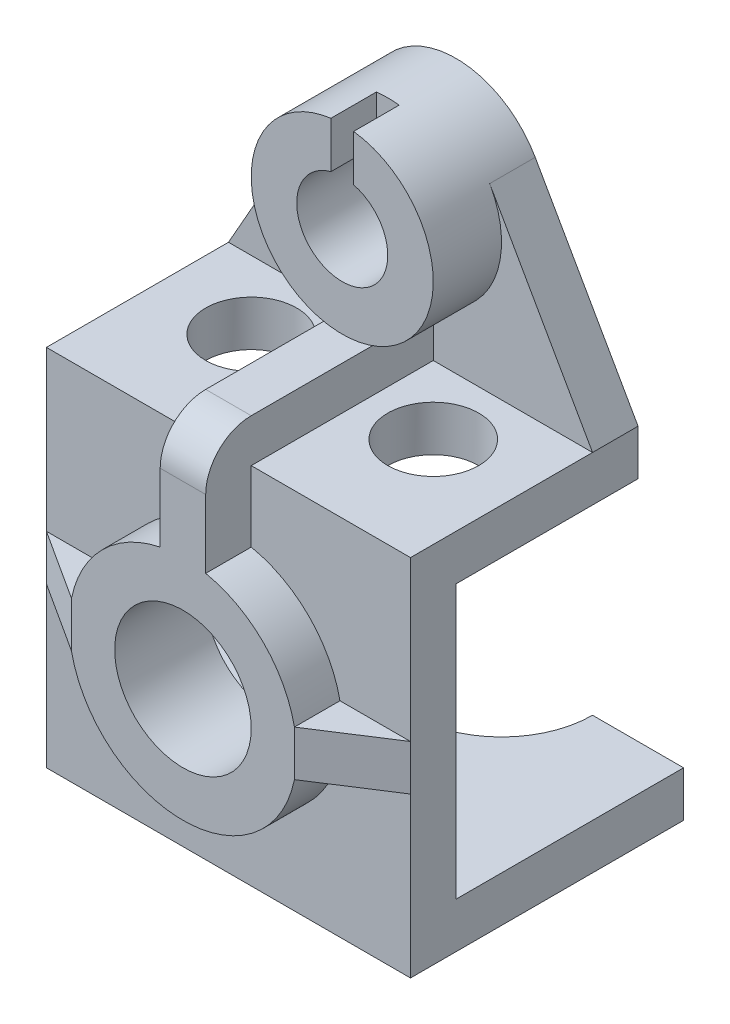
ISO-10303-21;
HEADER;
FILE_DESCRIPTION(('STEP AP214'),'2;1');
FILE_NAME('part.step','',(''),(''),'','','');
FILE_SCHEMA(('AUTOMOTIVE_DESIGN { 1 0 10303 214 1 1 1 1 }'));
ENDSEC;
DATA;
#1=APPLICATION_CONTEXT('core data for automotive mechanical design processes');
#2=APPLICATION_PROTOCOL_DEFINITION('international standard','automotive_design',2000,#1);
#3=PRODUCT_CONTEXT('',#1,'mechanical');
#4=PRODUCT('Part','Part','',(#3));
#5=PRODUCT_RELATED_PRODUCT_CATEGORY('part','',(#4));
#6=PRODUCT_DEFINITION_FORMATION('','',#4);
#7=PRODUCT_DEFINITION_CONTEXT('part definition',#1,'design');
#8=PRODUCT_DEFINITION('design','',#6,#7);
#9=PRODUCT_DEFINITION_SHAPE('','',#8);
#10=(LENGTH_UNIT() NAMED_UNIT(*) SI_UNIT(.MILLI.,.METRE.));
#11=(NAMED_UNIT(*) PLANE_ANGLE_UNIT() SI_UNIT($,.RADIAN.));
#12=(NAMED_UNIT(*) SI_UNIT($,.STERADIAN.) SOLID_ANGLE_UNIT());
#13=UNCERTAINTY_MEASURE_WITH_UNIT(LENGTH_MEASURE(1.E-05),#10,'distance_accuracy_value','');
#14=(GEOMETRIC_REPRESENTATION_CONTEXT(3) GLOBAL_UNCERTAINTY_ASSIGNED_CONTEXT((#13)) GLOBAL_UNIT_ASSIGNED_CONTEXT((#10,
#11,#12)) REPRESENTATION_CONTEXT('',''));
#15=CARTESIAN_POINT('',(0.,0.,0.));
#16=DIRECTION('',(0.,0.,1.));
#17=DIRECTION('',(1.,0.,0.));
#18=AXIS2_PLACEMENT_3D('',#15,#16,#17);
#19=CARTESIAN_POINT('',(-80.,9.99999999999999,0.));
#20=DIRECTION('',(0.,0.,-1.));
#21=DIRECTION('',(-1.,0.,0.));
#22=AXIS2_PLACEMENT_3D('',#19,#20,#21);
#23=PLANE('',#22);
#24=DIRECTION('',(0.,1.,0.));
#25=VECTOR('',#24,1.);
#26=CARTESIAN_POINT('',(-60.,0.,0.));
#27=LINE('',#26,#25);
#28=CARTESIAN_POINT('',(-60.,0.,0.));
#29=VERTEX_POINT('',#28);
#30=CARTESIAN_POINT('',(-60.,9.99999999999999,0.));
#31=VERTEX_POINT('',#30);
#32=EDGE_CURVE('E56',#29,#31,#27,.T.);
#33=ORIENTED_EDGE('',*,*,#32,.F.);
#34=DIRECTION('',(1.,0.,0.));
#35=VECTOR('',#34,1.);
#36=CARTESIAN_POINT('',(-80.,0.,0.));
#37=LINE('',#36,#35);
#38=CARTESIAN_POINT('',(-80.,0.,0.));
#39=VERTEX_POINT('',#38);
#40=EDGE_CURVE('E251',#39,#29,#37,.T.);
#41=ORIENTED_EDGE('',*,*,#40,.F.);
#42=DIRECTION('',(0.,1.,0.));
#43=VECTOR('',#42,1.);
#44=CARTESIAN_POINT('',(-80.,9.99999999999999,0.));
#45=LINE('',#44,#43);
#46=CARTESIAN_POINT('',(-80.,9.99999999999999,0.));
#47=VERTEX_POINT('',#46);
#48=EDGE_CURVE('E425',#39,#47,#45,.T.);
#49=ORIENTED_EDGE('',*,*,#48,.T.);
#50=DIRECTION('',(1.,0.,0.));
#51=VECTOR('',#50,1.);
#52=CARTESIAN_POINT('',(-80.,9.99999999999999,0.));
#53=LINE('',#52,#51);
#54=EDGE_CURVE('E276',#47,#31,#53,.T.);
#55=ORIENTED_EDGE('',*,*,#54,.T.);
#56=EDGE_LOOP('',(#33,#41,#49,#55));
#57=FACE_BOUND('',#56,.T.);
#58=ADVANCED_FACE('F44',(#57),#23,.T.);
#59=CARTESIAN_POINT('',(-40.,110.,35.));
#60=DIRECTION('',(0.,0.,-1.));
#61=DIRECTION('',(-1.,0.,0.));
#62=AXIS2_PLACEMENT_3D('',#59,#60,#61);
#63=CYLINDRICAL_SURFACE('',#62,20.);
#64=DIRECTION('',(0.,0.,-1.));
#65=VECTOR('',#64,1.);
#66=CARTESIAN_POINT('',(-57.398181667894,119.864242223859,20.));
#67=LINE('',#66,#65);
#68=CARTESIAN_POINT('',(-57.398181667894,119.864242223859,20.));
#69=VERTEX_POINT('',#68);
#70=CARTESIAN_POINT('',(-57.398181667894,119.864242223859,9.99999999999999));
#71=VERTEX_POINT('',#70);
#72=EDGE_CURVE('E415',#69,#71,#67,.T.);
#73=ORIENTED_EDGE('',*,*,#72,.F.);
#74=CARTESIAN_POINT('',(-40.,110.,20.));
#75=DIRECTION('',(0.,0.,-1.));
#76=DIRECTION('',(-1.,0.,0.));
#77=AXIS2_PLACEMENT_3D('',#74,#75,#76);
#78=CIRCLE('',#77,20.);
#79=CARTESIAN_POINT('',(-22.601818332106,119.864242223859,20.));
#80=VERTEX_POINT('',#79);
#81=EDGE_CURVE('E393',#80,#69,#78,.T.);
#82=ORIENTED_EDGE('',*,*,#81,.F.);
#83=DIRECTION('',(0.,0.,-1.));
#84=VECTOR('',#83,1.);
#85=CARTESIAN_POINT('',(-22.601818332106,119.864242223859,20.));
#86=LINE('',#85,#84);
#87=CARTESIAN_POINT('',(-22.601818332106,119.864242223859,9.99999999999999));
#88=VERTEX_POINT('',#87);
#89=EDGE_CURVE('E410',#80,#88,#86,.T.);
#90=ORIENTED_EDGE('',*,*,#89,.T.);
#91=CARTESIAN_POINT('',(-40.,110.,9.99999999999999));
#92=DIRECTION('',(0.,0.,-1.));
#93=DIRECTION('',(-1.,0.,0.));
#94=AXIS2_PLACEMENT_3D('',#91,#92,#93);
#95=CIRCLE('',#94,20.);
#96=EDGE_CURVE('E380',#71,#88,#95,.T.);
#97=ORIENTED_EDGE('',*,*,#96,.F.);
#98=EDGE_LOOP('',(#73,#82,#90,#97));
#99=FACE_BOUND('',#98,.T.);
#100=CARTESIAN_POINT('',(-40.,110.,35.));
#101=DIRECTION('',(0.,0.,-1.));
#102=DIRECTION('',(-1.,0.,0.));
#103=AXIS2_PLACEMENT_3D('',#100,#101,#102);
#104=CIRCLE('',#103,20.);
#105=CARTESIAN_POINT('',(-37.5000000000001,129.843134832984,35.));
#106=VERTEX_POINT('',#105);
#107=CARTESIAN_POINT('',(-42.5,129.843134832984,35.));
#108=VERTEX_POINT('',#107);
#109=EDGE_CURVE('E390',#106,#108,#104,.T.);
#110=ORIENTED_EDGE('',*,*,#109,.T.);
#111=DIRECTION('',(0.,0.,1.));
#112=VECTOR('',#111,1.);
#113=CARTESIAN_POINT('',(-42.5,129.843134832984,25.));
#114=LINE('',#113,#112);
#115=CARTESIAN_POINT('',(-42.5,129.843134832984,25.));
#116=VERTEX_POINT('',#115);
#117=EDGE_CURVE('E506',#116,#108,#114,.T.);
#118=ORIENTED_EDGE('',*,*,#117,.F.);
#119=CARTESIAN_POINT('',(-40.,110.,25.));
#120=DIRECTION('',(0.,0.,1.));
#121=DIRECTION('',(1.,0.,0.));
#122=AXIS2_PLACEMENT_3D('',#119,#120,#121);
#123=CIRCLE('',#122,20.);
#124=CARTESIAN_POINT('',(-37.5000000000001,129.843134832984,25.));
#125=VERTEX_POINT('',#124);
#126=EDGE_CURVE('E496',#125,#116,#123,.T.);
#127=ORIENTED_EDGE('',*,*,#126,.F.);
#128=DIRECTION('',(0.,0.,1.));
#129=VECTOR('',#128,1.);
#130=CARTESIAN_POINT('',(-37.5000000000001,129.843134832984,25.));
#131=LINE('',#130,#129);
#132=EDGE_CURVE('E507',#125,#106,#131,.T.);
#133=ORIENTED_EDGE('',*,*,#132,.T.);
#134=EDGE_LOOP('',(#110,#118,#127,#133));
#135=FACE_BOUND('',#134,.T.);
#136=ADVANCED_FACE('F566',(#99,#135),#63,.T.);
#137=CARTESIAN_POINT('',(0.,0.,35.));
#138=DIRECTION('',(0.,0.,-1.));
#139=DIRECTION('',(-1.,0.,0.));
#140=AXIS2_PLACEMENT_3D('',#137,#138,#139);
#141=PLANE('',#140);
#142=DIRECTION('',(0.,1.,0.));
#143=VECTOR('',#142,1.);
#144=CARTESIAN_POINT('',(-42.5000000000002,0.,35.));
#145=LINE('',#144,#143);
#146=CARTESIAN_POINT('',(-42.5,119.682458365519,35.));
#147=VERTEX_POINT('',#146);
#148=EDGE_CURVE('E487',#147,#108,#145,.T.);
#149=ORIENTED_EDGE('',*,*,#148,.T.);
#150=ORIENTED_EDGE('',*,*,#109,.F.);
#151=DIRECTION('',(0.,1.,0.));
#152=VECTOR('',#151,1.);
#153=CARTESIAN_POINT('',(-37.4999999999997,-1.02437479327167E-13,35.));
#154=LINE('',#153,#152);
#155=CARTESIAN_POINT('',(-37.5,119.682458365519,35.));
#156=VERTEX_POINT('',#155);
#157=EDGE_CURVE('E481',#156,#106,#154,.T.);
#158=ORIENTED_EDGE('',*,*,#157,.F.);
#159=CARTESIAN_POINT('',(-40.,110.,35.));
#160=DIRECTION('',(0.,0.,1.));
#161=DIRECTION('',(1.,0.,0.));
#162=AXIS2_PLACEMENT_3D('',#159,#160,#161);
#163=CIRCLE('',#162,10.);
#164=EDGE_CURVE('E504',#147,#156,#163,.T.);
#165=ORIENTED_EDGE('',*,*,#164,.F.);
#166=EDGE_LOOP('',(#149,#150,#158,#165));
#167=FACE_BOUND('',#166,.T.);
#168=ADVANCED_FACE('F637',(#167),#141,.F.);
#169=CARTESIAN_POINT('',(-40.,110.,0.));
#170=DIRECTION('',(0.,0.,1.));
#171=DIRECTION('',(1.,0.,0.));
#172=AXIS2_PLACEMENT_3D('',#169,#170,#171);
#173=CYLINDRICAL_SURFACE('',#172,10.);
#174=CARTESIAN_POINT('',(-40.,110.,9.99999999999999));
#175=DIRECTION('',(0.,0.,-1.));
#176=DIRECTION('',(-1.,0.,0.));
#177=AXIS2_PLACEMENT_3D('',#174,#175,#176);
#178=CIRCLE('',#177,10.);
#179=CARTESIAN_POINT('',(-50.,110.,9.99999999999999));
#180=VERTEX_POINT('',#179);
#181=EDGE_CURVE('E511',#180,#180,#178,.T.);
#182=ORIENTED_EDGE('',*,*,#181,.T.);
#183=EDGE_LOOP('',(#182));
#184=FACE_BOUND('',#183,.T.);
#185=DIRECTION('',(0.,0.,1.));
#186=VECTOR('',#185,1.);
#187=CARTESIAN_POINT('',(-42.5,119.682458365519,25.));
#188=LINE('',#187,#186);
#189=CARTESIAN_POINT('',(-42.5,119.682458365519,25.));
#190=VERTEX_POINT('',#189);
#191=EDGE_CURVE('E70',#190,#147,#188,.T.);
#192=ORIENTED_EDGE('',*,*,#191,.T.);
#193=ORIENTED_EDGE('',*,*,#164,.T.);
#194=DIRECTION('',(0.,0.,1.));
#195=VECTOR('',#194,1.);
#196=CARTESIAN_POINT('',(-37.5,119.682458365519,25.));
#197=LINE('',#196,#195);
#198=CARTESIAN_POINT('',(-37.5,119.682458365519,25.));
#199=VERTEX_POINT('',#198);
#200=EDGE_CURVE('E499',#199,#156,#197,.T.);
#201=ORIENTED_EDGE('',*,*,#200,.F.);
#202=CARTESIAN_POINT('',(-40.,110.,25.));
#203=DIRECTION('',(0.,0.,1.));
#204=DIRECTION('',(1.,0.,0.));
#205=AXIS2_PLACEMENT_3D('',#202,#203,#204);
#206=CIRCLE('',#205,10.);
#207=EDGE_CURVE('E489',#199,#190,#206,.T.);
#208=ORIENTED_EDGE('',*,*,#207,.T.);
#209=EDGE_LOOP('',(#192,#193,#201,#208));
#210=FACE_BOUND('',#209,.T.);
#211=ADVANCED_FACE('F681',(#184,#210),#173,.F.);
#212=CARTESIAN_POINT('',(-80.,0.,60.));
#213=DIRECTION('',(0.,0.,1.));
#214=DIRECTION('',(1.,0.,0.));
#215=AXIS2_PLACEMENT_3D('',#212,#213,#214);
#216=PLANE('',#215);
#217=DIRECTION('',(-1.,0.,0.));
#218=VECTOR('',#217,1.);
#219=CARTESIAN_POINT('',(-64.4948974278318,35.,60.));
#220=LINE('',#219,#218);
#221=CARTESIAN_POINT('',(-64.4948974278318,35.,60.));
#222=VERTEX_POINT('',#221);
#223=CARTESIAN_POINT('',(-80.,35.,60.));
#224=VERTEX_POINT('',#223);
#225=EDGE_CURVE('E340',#222,#224,#220,.T.);
#226=ORIENTED_EDGE('',*,*,#225,.T.);
#227=DIRECTION('',(0.,-1.,0.));
#228=VECTOR('',#227,1.);
#229=CARTESIAN_POINT('',(-80.,0.,60.));
#230=LINE('',#229,#228);
#231=CARTESIAN_POINT('',(-80.,0.,60.));
#232=VERTEX_POINT('',#231);
#233=EDGE_CURVE('E442',#224,#232,#230,.T.);
#234=ORIENTED_EDGE('',*,*,#233,.T.);
#235=DIRECTION('',(1.,0.,0.));
#236=VECTOR('',#235,1.);
#237=CARTESIAN_POINT('',(-80.,0.,60.));
#238=LINE('',#237,#236);
#239=CARTESIAN_POINT('',(0.,0.,60.));
#240=VERTEX_POINT('',#239);
#241=EDGE_CURVE('E258',#232,#240,#238,.T.);
#242=ORIENTED_EDGE('',*,*,#241,.T.);
#243=DIRECTION('',(0.,-1.,0.));
#244=VECTOR('',#243,1.);
#245=CARTESIAN_POINT('',(0.,0.,60.));
#246=LINE('',#245,#244);
#247=CARTESIAN_POINT('',(0.,35.,60.));
#248=VERTEX_POINT('',#247);
#249=EDGE_CURVE('E465',#248,#240,#246,.T.);
#250=ORIENTED_EDGE('',*,*,#249,.F.);
#251=DIRECTION('',(-1.,0.,0.));
#252=VECTOR('',#251,1.);
#253=CARTESIAN_POINT('',(-15.5051025721682,35.,60.));
#254=LINE('',#253,#252);
#255=CARTESIAN_POINT('',(-15.5051025721682,35.,60.));
#256=VERTEX_POINT('',#255);
#257=EDGE_CURVE('E349',#248,#256,#254,.T.);
#258=ORIENTED_EDGE('',*,*,#257,.T.);
#259=CARTESIAN_POINT('',(-40.,40.,60.));
#260=DIRECTION('',(0.,0.,1.));
#261=DIRECTION('',(1.,0.,0.));
#262=AXIS2_PLACEMENT_3D('',#259,#260,#261);
#263=CIRCLE('',#262,25.);
#264=EDGE_CURVE('E421',#222,#256,#263,.T.);
#265=ORIENTED_EDGE('',*,*,#264,.F.);
#266=EDGE_LOOP('',(#226,#234,#242,#250,#258,#265));
#267=FACE_BOUND('',#266,.T.);
#268=ADVANCED_FACE('F477',(#267),#216,.T.);
#269=CARTESIAN_POINT('',(-40.,40.,70.));
#270=DIRECTION('',(0.,0.,-1.));
#271=DIRECTION('',(-1.,0.,0.));
#272=AXIS2_PLACEMENT_3D('',#269,#270,#271);
#273=CYLINDRICAL_SURFACE('',#272,25.);
#274=CARTESIAN_POINT('',(-40.,40.,70.));
#275=DIRECTION('',(0.,0.,1.));
#276=DIRECTION('',(1.,0.,0.));
#277=AXIS2_PLACEMENT_3D('',#274,#275,#276);
#278=CIRCLE('',#277,25.);
#279=CARTESIAN_POINT('',(-64.4948974278318,35.,70.));
#280=VERTEX_POINT('',#279);
#281=CARTESIAN_POINT('',(-15.5051025721682,35.,70.));
#282=VERTEX_POINT('',#281);
#283=EDGE_CURVE('E416',#280,#282,#278,.T.);
#284=ORIENTED_EDGE('',*,*,#283,.F.);
#285=DIRECTION('',(0.,0.,1.));
#286=VECTOR('',#285,1.);
#287=CARTESIAN_POINT('',(-64.4948974278318,35.,-0.002000000000002));
#288=LINE('',#287,#286);
#289=EDGE_CURVE('E329',#222,#280,#288,.T.);
#290=ORIENTED_EDGE('',*,*,#289,.F.);
#291=ORIENTED_EDGE('',*,*,#264,.T.);
#292=DIRECTION('',(0.,0.,1.));
#293=VECTOR('',#292,1.);
#294=CARTESIAN_POINT('',(-15.5051025721682,35.,-0.002000000000002));
#295=LINE('',#294,#293);
#296=EDGE_CURVE('E345',#256,#282,#295,.T.);
#297=ORIENTED_EDGE('',*,*,#296,.T.);
#298=EDGE_LOOP('',(#284,#290,#291,#297));
#299=FACE_BOUND('',#298,.T.);
#300=ADVANCED_FACE('F594',(#299),#273,.T.);
#301=DIRECTION('',(1.,0.,0.));
#302=VECTOR('',#301,1.);
#303=CARTESIAN_POINT('',(-64.4948974278318,45.,60.));
#304=LINE('',#303,#302);
#305=CARTESIAN_POINT('',(-80.,45.,60.));
#306=VERTEX_POINT('',#305);
#307=CARTESIAN_POINT('',(-64.4948974278318,45.,60.));
#308=VERTEX_POINT('',#307);
#309=EDGE_CURVE('E334',#306,#308,#304,.T.);
#310=ORIENTED_EDGE('',*,*,#309,.T.);
#311=CARTESIAN_POINT('',(-45.,64.4948974278318,60.));
#312=VERTEX_POINT('',#311);
#313=EDGE_CURVE('E289',#312,#308,#263,.T.);
#314=ORIENTED_EDGE('',*,*,#313,.F.);
#315=DIRECTION('',(0.,1.,0.));
#316=VECTOR('',#315,1.);
#317=CARTESIAN_POINT('',(-45.,-0.002000000000002,60.));
#318=LINE('',#317,#316);
#319=CARTESIAN_POINT('',(-45.,80.,60.));
#320=VERTEX_POINT('',#319);
#321=EDGE_CURVE('E355',#312,#320,#318,.T.);
#322=ORIENTED_EDGE('',*,*,#321,.T.);
#323=DIRECTION('',(1.,0.,0.));
#324=VECTOR('',#323,1.);
#325=CARTESIAN_POINT('',(-80.,80.,60.));
#326=LINE('',#325,#324);
#327=CARTESIAN_POINT('',(-80.,80.,60.));
#328=VERTEX_POINT('',#327);
#329=EDGE_CURVE('E264',#328,#320,#326,.T.);
#330=ORIENTED_EDGE('',*,*,#329,.F.);
#331=EDGE_CURVE('E443',#328,#306,#230,.T.);
#332=ORIENTED_EDGE('',*,*,#331,.T.);
#333=EDGE_LOOP('',(#310,#314,#322,#330,#332));
#334=FACE_BOUND('',#333,.T.);
#335=ADVANCED_FACE('F608',(#334),#216,.T.);
#336=ORIENTED_EDGE('',*,*,#313,.T.);
#337=DIRECTION('',(0.,0.,1.));
#338=VECTOR('',#337,1.);
#339=CARTESIAN_POINT('',(-64.4948974278318,45.,-0.002000000000002));
#340=LINE('',#339,#338);
#341=CARTESIAN_POINT('',(-64.4948974278318,45.,70.));
#342=VERTEX_POINT('',#341);
#343=EDGE_CURVE('E332',#308,#342,#340,.T.);
#344=ORIENTED_EDGE('',*,*,#343,.T.);
#345=CARTESIAN_POINT('',(-45.,64.4948974278318,70.));
#346=VERTEX_POINT('',#345);
#347=EDGE_CURVE('E419',#346,#342,#278,.T.);
#348=ORIENTED_EDGE('',*,*,#347,.F.);
#349=DIRECTION('',(0.,0.,-1.));
#350=VECTOR('',#349,1.);
#351=CARTESIAN_POINT('',(-45.,64.4948974278318,70.));
#352=LINE('',#351,#350);
#353=EDGE_CURVE('E343',#346,#312,#352,.T.);
#354=ORIENTED_EDGE('',*,*,#353,.T.);
#355=EDGE_LOOP('',(#336,#344,#348,#354));
#356=FACE_BOUND('',#355,.T.);
#357=ADVANCED_FACE('F615',(#356),#273,.T.);
#358=DIRECTION('',(1.,0.,0.));
#359=VECTOR('',#358,1.);
#360=CARTESIAN_POINT('',(-15.5051025721682,45.,60.));
#361=LINE('',#360,#359);
#362=CARTESIAN_POINT('',(-15.5051025721682,45.,60.));
#363=VERTEX_POINT('',#362);
#364=CARTESIAN_POINT('',(0.,45.,60.));
#365=VERTEX_POINT('',#364);
#366=EDGE_CURVE('E347',#363,#365,#361,.T.);
#367=ORIENTED_EDGE('',*,*,#366,.T.);
#368=CARTESIAN_POINT('',(0.,80.,60.));
#369=VERTEX_POINT('',#368);
#370=EDGE_CURVE('E461',#369,#365,#246,.T.);
#371=ORIENTED_EDGE('',*,*,#370,.F.);
#372=CARTESIAN_POINT('',(-35.,80.,60.));
#373=VERTEX_POINT('',#372);
#374=EDGE_CURVE('E275',#373,#369,#326,.T.);
#375=ORIENTED_EDGE('',*,*,#374,.F.);
#376=DIRECTION('',(0.,1.,0.));
#377=VECTOR('',#376,1.);
#378=CARTESIAN_POINT('',(-35.,-0.002000000000002,60.));
#379=LINE('',#378,#377);
#380=CARTESIAN_POINT('',(-35.,64.4948974278318,60.));
#381=VERTEX_POINT('',#380);
#382=EDGE_CURVE('E358',#381,#373,#379,.T.);
#383=ORIENTED_EDGE('',*,*,#382,.F.);
#384=EDGE_CURVE('E265',#363,#381,#263,.T.);
#385=ORIENTED_EDGE('',*,*,#384,.F.);
#386=EDGE_LOOP('',(#367,#371,#375,#383,#385));
#387=FACE_BOUND('',#386,.T.);
#388=ADVANCED_FACE('F572',(#387),#216,.T.);
#389=CARTESIAN_POINT('',(-15.5051025721682,45.,70.));
#390=VERTEX_POINT('',#389);
#391=CARTESIAN_POINT('',(-35.,64.4948974278318,70.));
#392=VERTEX_POINT('',#391);
#393=EDGE_CURVE('E411',#390,#392,#278,.T.);
#394=ORIENTED_EDGE('',*,*,#393,.F.);
#395=DIRECTION('',(0.,0.,1.));
#396=VECTOR('',#395,1.);
#397=CARTESIAN_POINT('',(-15.5051025721682,45.,-0.002000000000002));
#398=LINE('',#397,#396);
#399=EDGE_CURVE('E337',#363,#390,#398,.T.);
#400=ORIENTED_EDGE('',*,*,#399,.F.);
#401=ORIENTED_EDGE('',*,*,#384,.T.);
#402=DIRECTION('',(0.,0.,-1.));
#403=VECTOR('',#402,1.);
#404=CARTESIAN_POINT('',(-35.,64.4948974278318,70.));
#405=LINE('',#404,#403);
#406=EDGE_CURVE('E357',#381,#392,#405,.F.);
#407=ORIENTED_EDGE('',*,*,#406,.T.);
#408=EDGE_LOOP('',(#394,#400,#401,#407));
#409=FACE_BOUND('',#408,.T.);
#410=ADVANCED_FACE('F529',(#409),#273,.T.);
#411=CARTESIAN_POINT('',(-80.,80.,60.));
#412=DIRECTION('',(0.,1.,0.));
#413=DIRECTION('',(0.,0.,1.));
#414=AXIS2_PLACEMENT_3D('',#411,#412,#413);
#415=PLANE('',#414);
#416=CARTESIAN_POINT('',(-60.,80.,35.));
#417=DIRECTION('',(0.,1.,0.));
#418=DIRECTION('',(0.,0.,1.));
#419=AXIS2_PLACEMENT_3D('',#416,#417,#418);
#420=CIRCLE('',#419,10.);
#421=CARTESIAN_POINT('',(-60.,80.,45.));
#422=VERTEX_POINT('',#421);
#423=EDGE_CURVE('E307',#422,#422,#420,.T.);
#424=ORIENTED_EDGE('',*,*,#423,.F.);
#425=EDGE_LOOP('',(#424));
#426=FACE_BOUND('',#425,.T.);
#427=DIRECTION('',(0.,0.,1.));
#428=VECTOR('',#427,1.);
#429=CARTESIAN_POINT('',(-45.,80.,-0.002000000000002));
#430=LINE('',#429,#428);
#431=CARTESIAN_POINT('',(-45.,80.,20.));
#432=VERTEX_POINT('',#431);
#433=EDGE_CURVE('E369',#432,#320,#430,.T.);
#434=ORIENTED_EDGE('',*,*,#433,.F.);
#435=DIRECTION('',(1.,0.,0.));
#436=VECTOR('',#435,1.);
#437=CARTESIAN_POINT('',(0.,80.,20.));
#438=LINE('',#437,#436);
#439=CARTESIAN_POINT('',(-80.,80.,20.));
#440=VERTEX_POINT('',#439);
#441=EDGE_CURVE('E402',#440,#432,#438,.T.);
#442=ORIENTED_EDGE('',*,*,#441,.F.);
#443=DIRECTION('',(0.,0.,1.));
#444=VECTOR('',#443,1.);
#445=CARTESIAN_POINT('',(-80.,80.,60.));
#446=LINE('',#445,#444);
#447=EDGE_CURVE('E437',#440,#328,#446,.T.);
#448=ORIENTED_EDGE('',*,*,#447,.T.);
#449=ORIENTED_EDGE('',*,*,#329,.T.);
#450=EDGE_LOOP('',(#434,#442,#448,#449));
#451=FACE_BOUND('',#450,.T.);
#452=ADVANCED_FACE('F524',(#426,#451),#415,.T.);
#453=DIRECTION('',(0.,1.,0.));
#454=VECTOR('',#453,1.);
#455=CARTESIAN_POINT('',(-20.,0.,0.));
#456=LINE('',#455,#454);
#457=CARTESIAN_POINT('',(-20.,9.99999999999999,0.));
#458=VERTEX_POINT('',#457);
#459=CARTESIAN_POINT('',(-20.,0.,0.));
#460=VERTEX_POINT('',#459);
#461=EDGE_CURVE('E237',#458,#460,#456,.F.);
#462=ORIENTED_EDGE('',*,*,#461,.F.);
#463=CARTESIAN_POINT('',(0.,9.99999999999999,0.));
#464=VERTEX_POINT('',#463);
#465=EDGE_CURVE('E285',#458,#464,#53,.T.);
#466=ORIENTED_EDGE('',*,*,#465,.T.);
#467=DIRECTION('',(0.,1.,0.));
#468=VECTOR('',#467,1.);
#469=CARTESIAN_POINT('',(0.,9.99999999999999,0.));
#470=LINE('',#469,#468);
#471=CARTESIAN_POINT('',(0.,0.,0.));
#472=VERTEX_POINT('',#471);
#473=EDGE_CURVE('E259',#472,#464,#470,.T.);
#474=ORIENTED_EDGE('',*,*,#473,.F.);
#475=EDGE_CURVE('E252',#460,#472,#37,.T.);
#476=ORIENTED_EDGE('',*,*,#475,.F.);
#477=EDGE_LOOP('',(#462,#466,#474,#476));
#478=FACE_BOUND('',#477,.T.);
#479=ADVANCED_FACE('F257',(#478),#23,.T.);
#480=CARTESIAN_POINT('',(-80.,0.,0.));
#481=DIRECTION('',(0.,-1.,0.));
#482=DIRECTION('',(0.,0.,-1.));
#483=AXIS2_PLACEMENT_3D('',#480,#481,#482);
#484=PLANE('',#483);
#485=CARTESIAN_POINT('',(-40.,0.,0.));
#486=DIRECTION('',(0.,1.,0.));
#487=DIRECTION('',(0.,0.,1.));
#488=AXIS2_PLACEMENT_3D('',#485,#486,#487);
#489=CIRCLE('',#488,20.);
#490=EDGE_CURVE('E245',#29,#460,#489,.T.);
#491=ORIENTED_EDGE('',*,*,#490,.T.);
#492=ORIENTED_EDGE('',*,*,#475,.T.);
#493=DIRECTION('',(0.,0.,-1.));
#494=VECTOR('',#493,1.);
#495=CARTESIAN_POINT('',(0.,0.,0.));
#496=LINE('',#495,#494);
#497=EDGE_CURVE('E269',#240,#472,#496,.T.);
#498=ORIENTED_EDGE('',*,*,#497,.F.);
#499=ORIENTED_EDGE('',*,*,#241,.F.);
#500=DIRECTION('',(0.,0.,-1.));
#501=VECTOR('',#500,1.);
#502=CARTESIAN_POINT('',(-80.,0.,0.));
#503=LINE('',#502,#501);
#504=EDGE_CURVE('E450',#232,#39,#503,.T.);
#505=ORIENTED_EDGE('',*,*,#504,.T.);
#506=ORIENTED_EDGE('',*,*,#40,.T.);
#507=EDGE_LOOP('',(#491,#492,#498,#499,#505,#506));
#508=FACE_BOUND('',#507,.T.);
#509=ADVANCED_FACE('F248',(#508),#484,.T.);
#510=CARTESIAN_POINT('',(-20.,80.,35.));
#511=DIRECTION('',(0.,1.,0.));
#512=DIRECTION('',(0.,0.,1.));
#513=AXIS2_PLACEMENT_3D('',#510,#511,#512);
#514=CIRCLE('',#513,10.);
#515=CARTESIAN_POINT('',(-20.,80.,45.));
#516=VERTEX_POINT('',#515);
#517=EDGE_CURVE('E294',#516,#516,#514,.T.);
#518=ORIENTED_EDGE('',*,*,#517,.F.);
#519=EDGE_LOOP('',(#518));
#520=FACE_BOUND('',#519,.T.);
#521=DIRECTION('',(0.,0.,1.));
#522=VECTOR('',#521,1.);
#523=CARTESIAN_POINT('',(-35.,80.,-0.002000000000002));
#524=LINE('',#523,#522);
#525=CARTESIAN_POINT('',(-35.,80.,20.));
#526=VERTEX_POINT('',#525);
#527=EDGE_CURVE('E379',#526,#373,#524,.T.);
#528=ORIENTED_EDGE('',*,*,#527,.T.);
#529=ORIENTED_EDGE('',*,*,#374,.T.);
#530=DIRECTION('',(0.,0.,1.));
#531=VECTOR('',#530,1.);
#532=CARTESIAN_POINT('',(0.,80.,60.));
#533=LINE('',#532,#531);
#534=CARTESIAN_POINT('',(0.,80.,20.));
#535=VERTEX_POINT('',#534);
#536=EDGE_CURVE('E463',#535,#369,#533,.T.);
#537=ORIENTED_EDGE('',*,*,#536,.F.);
#538=EDGE_CURVE('E396',#526,#535,#438,.T.);
#539=ORIENTED_EDGE('',*,*,#538,.F.);
#540=EDGE_LOOP('',(#528,#529,#537,#539));
#541=FACE_BOUND('',#540,.T.);
#542=ADVANCED_FACE('F530',(#520,#541),#415,.T.);
#543=CARTESIAN_POINT('',(-80.,80.,9.99999999999999));
#544=DIRECTION('',(0.,0.,-1.));
#545=DIRECTION('',(-1.,0.,0.));
#546=AXIS2_PLACEMENT_3D('',#543,#544,#545);
#547=PLANE('',#546);
#548=ORIENTED_EDGE('',*,*,#181,.F.);
#549=EDGE_LOOP('',(#548));
#550=FACE_BOUND('',#549,.T.);
#551=DIRECTION('',(0.,1.,0.));
#552=VECTOR('',#551,1.);
#553=CARTESIAN_POINT('',(0.,80.,9.99999999999999));
#554=LINE('',#553,#552);
#555=CARTESIAN_POINT('',(0.,70.,9.99999999999999));
#556=VERTEX_POINT('',#555);
#557=CARTESIAN_POINT('',(0.,80.,9.99999999999999));
#558=VERTEX_POINT('',#557);
#559=EDGE_CURVE('E459',#556,#558,#554,.T.);
#560=ORIENTED_EDGE('',*,*,#559,.F.);
#561=DIRECTION('',(1.,0.,0.));
#562=VECTOR('',#561,1.);
#563=CARTESIAN_POINT('',(-80.,70.,9.99999999999999));
#564=LINE('',#563,#562);
#565=CARTESIAN_POINT('',(-80.,70.,9.99999999999999));
#566=VERTEX_POINT('',#565);
#567=EDGE_CURVE('E271',#566,#556,#564,.T.);
#568=ORIENTED_EDGE('',*,*,#567,.F.);
#569=DIRECTION('',(0.,1.,0.));
#570=VECTOR('',#569,1.);
#571=CARTESIAN_POINT('',(-80.,80.,9.99999999999999));
#572=LINE('',#571,#570);
#573=CARTESIAN_POINT('',(-80.,80.,9.99999999999999));
#574=VERTEX_POINT('',#573);
#575=EDGE_CURVE('E436',#566,#574,#572,.T.);
#576=ORIENTED_EDGE('',*,*,#575,.T.);
#577=DIRECTION('',(-0.493212111192934,-0.869909083394701,0.));
#578=VECTOR('',#577,1.);
#579=CARTESIAN_POINT('',(-94.8633207151696,53.7846305755521,9.99999999999999));
#580=LINE('',#579,#578);
#581=EDGE_CURVE('E399',#71,#574,#580,.T.);
#582=ORIENTED_EDGE('',*,*,#581,.F.);
#583=ORIENTED_EDGE('',*,*,#96,.T.);
#584=DIRECTION('',(0.493212111192934,-0.869909083394701,0.));
#585=VECTOR('',#584,1.);
#586=CARTESIAN_POINT('',(34.3239756453608,19.4606549301913,9.99999999999999));
#587=LINE('',#586,#585);
#588=EDGE_CURVE('E388',#88,#558,#587,.T.);
#589=ORIENTED_EDGE('',*,*,#588,.T.);
#590=EDGE_LOOP('',(#560,#568,#576,#582,#583,#589));
#591=FACE_BOUND('',#590,.T.);
#592=ADVANCED_FACE('F550',(#550,#591),#547,.T.);
#593=CARTESIAN_POINT('',(-80.,70.,9.99999999999999));
#594=DIRECTION('',(0.,-1.,0.));
#595=DIRECTION('',(0.,0.,-1.));
#596=AXIS2_PLACEMENT_3D('',#593,#594,#595);
#597=PLANE('',#596);
#598=CARTESIAN_POINT('',(-20.,70.,35.));
#599=DIRECTION('',(0.,-1.,0.));
#600=DIRECTION('',(0.,0.,-1.));
#601=AXIS2_PLACEMENT_3D('',#598,#599,#600);
#602=CIRCLE('',#601,10.);
#603=CARTESIAN_POINT('',(-20.,70.,25.));
#604=VERTEX_POINT('',#603);
#605=EDGE_CURVE('E295',#604,#604,#602,.T.);
#606=ORIENTED_EDGE('',*,*,#605,.F.);
#607=EDGE_LOOP('',(#606));
#608=FACE_BOUND('',#607,.T.);
#609=CARTESIAN_POINT('',(-60.,70.,35.));
#610=DIRECTION('',(0.,-1.,0.));
#611=DIRECTION('',(0.,0.,-1.));
#612=AXIS2_PLACEMENT_3D('',#609,#610,#611);
#613=CIRCLE('',#612,10.);
#614=CARTESIAN_POINT('',(-60.,70.,25.));
#615=VERTEX_POINT('',#614);
#616=EDGE_CURVE('E292',#615,#615,#613,.T.);
#617=ORIENTED_EDGE('',*,*,#616,.F.);
#618=EDGE_LOOP('',(#617));
#619=FACE_BOUND('',#618,.T.);
#620=DIRECTION('',(0.,0.,-1.));
#621=VECTOR('',#620,1.);
#622=CARTESIAN_POINT('',(0.,70.,9.99999999999999));
#623=LINE('',#622,#621);
#624=CARTESIAN_POINT('',(0.,70.,50.));
#625=VERTEX_POINT('',#624);
#626=EDGE_CURVE('E457',#625,#556,#623,.T.);
#627=ORIENTED_EDGE('',*,*,#626,.F.);
#628=DIRECTION('',(1.,0.,0.));
#629=VECTOR('',#628,1.);
#630=CARTESIAN_POINT('',(-80.,70.,50.));
#631=LINE('',#630,#629);
#632=CARTESIAN_POINT('',(-80.,70.,50.));
#633=VERTEX_POINT('',#632);
#634=EDGE_CURVE('E273',#633,#625,#631,.T.);
#635=ORIENTED_EDGE('',*,*,#634,.F.);
#636=DIRECTION('',(0.,0.,-1.));
#637=VECTOR('',#636,1.);
#638=CARTESIAN_POINT('',(-80.,70.,9.99999999999999));
#639=LINE('',#638,#637);
#640=EDGE_CURVE('E433',#633,#566,#639,.T.);
#641=ORIENTED_EDGE('',*,*,#640,.T.);
#642=ORIENTED_EDGE('',*,*,#567,.T.);
#643=EDGE_LOOP('',(#627,#635,#641,#642));
#644=FACE_BOUND('',#643,.T.);
#645=ADVANCED_FACE('F552',(#608,#619,#644),#597,.T.);
#646=CARTESIAN_POINT('',(-80.,70.,50.));
#647=DIRECTION('',(0.,0.,-1.));
#648=DIRECTION('',(-1.,0.,0.));
#649=AXIS2_PLACEMENT_3D('',#646,#647,#648);
#650=PLANE('',#649);
#651=CARTESIAN_POINT('',(-40.,40.,50.));
#652=DIRECTION('',(0.,0.,-1.));
#653=DIRECTION('',(-1.,0.,0.));
#654=AXIS2_PLACEMENT_3D('',#651,#652,#653);
#655=CIRCLE('',#654,15.);
#656=CARTESIAN_POINT('',(-55.,40.,50.));
#657=VERTEX_POINT('',#656);
#658=EDGE_CURVE('E301',#657,#657,#655,.T.);
#659=ORIENTED_EDGE('',*,*,#658,.F.);
#660=EDGE_LOOP('',(#659));
#661=FACE_BOUND('',#660,.T.);
#662=DIRECTION('',(0.,1.,0.));
#663=VECTOR('',#662,1.);
#664=CARTESIAN_POINT('',(0.,70.,50.));
#665=LINE('',#664,#663);
#666=CARTESIAN_POINT('',(0.,9.99999999999999,50.));
#667=VERTEX_POINT('',#666);
#668=EDGE_CURVE('E454',#667,#625,#665,.T.);
#669=ORIENTED_EDGE('',*,*,#668,.F.);
#670=DIRECTION('',(1.,0.,0.));
#671=VECTOR('',#670,1.);
#672=CARTESIAN_POINT('',(-80.,9.99999999999999,50.));
#673=LINE('',#672,#671);
#674=CARTESIAN_POINT('',(-80.,9.99999999999999,50.));
#675=VERTEX_POINT('',#674);
#676=EDGE_CURVE('E280',#675,#667,#673,.T.);
#677=ORIENTED_EDGE('',*,*,#676,.F.);
#678=DIRECTION('',(0.,1.,0.));
#679=VECTOR('',#678,1.);
#680=CARTESIAN_POINT('',(-80.,70.,50.));
#681=LINE('',#680,#679);
#682=EDGE_CURVE('E427',#675,#633,#681,.T.);
#683=ORIENTED_EDGE('',*,*,#682,.T.);
#684=ORIENTED_EDGE('',*,*,#634,.T.);
#685=EDGE_LOOP('',(#669,#677,#683,#684));
#686=FACE_BOUND('',#685,.T.);
#687=ADVANCED_FACE('F554',(#661,#686),#650,.T.);
#688=CARTESIAN_POINT('',(-80.,9.99999999999999,50.));
#689=DIRECTION('',(0.,1.,0.));
#690=DIRECTION('',(0.,0.,1.));
#691=AXIS2_PLACEMENT_3D('',#688,#689,#690);
#692=PLANE('',#691);
#693=CARTESIAN_POINT('',(-40.,9.99999999999999,0.));
#694=DIRECTION('',(0.,1.,0.));
#695=DIRECTION('',(0.,0.,1.));
#696=AXIS2_PLACEMENT_3D('',#693,#694,#695);
#697=CIRCLE('',#696,20.);
#698=EDGE_CURVE('E11',#31,#458,#697,.T.);
#699=ORIENTED_EDGE('',*,*,#698,.F.);
#700=ORIENTED_EDGE('',*,*,#54,.F.);
#701=DIRECTION('',(0.,0.,1.));
#702=VECTOR('',#701,1.);
#703=CARTESIAN_POINT('',(-80.,9.99999999999999,50.));
#704=LINE('',#703,#702);
#705=EDGE_CURVE('E430',#47,#675,#704,.T.);
#706=ORIENTED_EDGE('',*,*,#705,.T.);
#707=ORIENTED_EDGE('',*,*,#676,.T.);
#708=DIRECTION('',(0.,0.,1.));
#709=VECTOR('',#708,1.);
#710=CARTESIAN_POINT('',(0.,9.99999999999999,50.));
#711=LINE('',#710,#709);
#712=EDGE_CURVE('E448',#464,#667,#711,.T.);
#713=ORIENTED_EDGE('',*,*,#712,.F.);
#714=ORIENTED_EDGE('',*,*,#465,.F.);
#715=EDGE_LOOP('',(#699,#700,#706,#707,#713,#714));
#716=FACE_BOUND('',#715,.T.);
#717=ADVANCED_FACE('F556',(#716),#692,.T.);
#718=CARTESIAN_POINT('',(-80.,0.,0.));
#719=DIRECTION('',(-1.,0.,0.));
#720=DIRECTION('',(0.,0.,1.));
#721=AXIS2_PLACEMENT_3D('',#718,#719,#720);
#722=PLANE('',#721);
#723=DIRECTION('',(0.,1.,0.));
#724=VECTOR('',#723,1.);
#725=CARTESIAN_POINT('',(-80.,20.,60.));
#726=LINE('',#725,#724);
#727=EDGE_CURVE('E314',#224,#306,#726,.T.);
#728=ORIENTED_EDGE('',*,*,#727,.T.);
#729=ORIENTED_EDGE('',*,*,#331,.F.);
#730=ORIENTED_EDGE('',*,*,#447,.F.);
#731=EDGE_CURVE('E439',#574,#440,#446,.T.);
#732=ORIENTED_EDGE('',*,*,#731,.F.);
#733=ORIENTED_EDGE('',*,*,#575,.F.);
#734=ORIENTED_EDGE('',*,*,#640,.F.);
#735=ORIENTED_EDGE('',*,*,#682,.F.);
#736=ORIENTED_EDGE('',*,*,#705,.F.);
#737=ORIENTED_EDGE('',*,*,#48,.F.);
#738=ORIENTED_EDGE('',*,*,#504,.F.);
#739=ORIENTED_EDGE('',*,*,#233,.F.);
#740=EDGE_LOOP('',(#728,#729,#730,#732,#733,#734,#735,#736,#737,#738,#739));
#741=FACE_BOUND('',#740,.T.);
#742=ADVANCED_FACE('F483',(#741),#722,.T.);
#743=CARTESIAN_POINT('',(0.,0.,0.));
#744=DIRECTION('',(-1.,0.,0.));
#745=DIRECTION('',(0.,0.,1.));
#746=AXIS2_PLACEMENT_3D('',#743,#744,#745);
#747=PLANE('',#746);
#748=ORIENTED_EDGE('',*,*,#370,.T.);
#749=DIRECTION('',(0.,1.,0.));
#750=VECTOR('',#749,1.);
#751=CARTESIAN_POINT('',(0.,20.,60.));
#752=LINE('',#751,#750);
#753=EDGE_CURVE('E313',#248,#365,#752,.T.);
#754=ORIENTED_EDGE('',*,*,#753,.F.);
#755=ORIENTED_EDGE('',*,*,#249,.T.);
#756=ORIENTED_EDGE('',*,*,#497,.T.);
#757=ORIENTED_EDGE('',*,*,#473,.T.);
#758=ORIENTED_EDGE('',*,*,#712,.T.);
#759=ORIENTED_EDGE('',*,*,#668,.T.);
#760=ORIENTED_EDGE('',*,*,#626,.T.);
#761=ORIENTED_EDGE('',*,*,#559,.T.);
#762=EDGE_CURVE('E464',#558,#535,#533,.T.);
#763=ORIENTED_EDGE('',*,*,#762,.T.);
#764=ORIENTED_EDGE('',*,*,#536,.T.);
#765=EDGE_LOOP('',(#748,#754,#755,#756,#757,#758,#759,#760,#761,#763,#764));
#766=FACE_BOUND('',#765,.T.);
#767=ADVANCED_FACE('F475',(#766),#747,.F.);
#768=CARTESIAN_POINT('',(-40.,40.,70.));
#769=DIRECTION('',(0.,0.,1.));
#770=DIRECTION('',(1.,0.,0.));
#771=AXIS2_PLACEMENT_3D('',#768,#769,#770);
#772=PLANE('',#771);
#773=CARTESIAN_POINT('',(-40.,40.,70.));
#774=DIRECTION('',(0.,0.,1.));
#775=DIRECTION('',(1.,0.,0.));
#776=AXIS2_PLACEMENT_3D('',#773,#774,#775);
#777=CIRCLE('',#776,15.);
#778=CARTESIAN_POINT('',(-25.,40.,70.));
#779=VERTEX_POINT('',#778);
#780=EDGE_CURVE('E300',#779,#779,#777,.T.);
#781=ORIENTED_EDGE('',*,*,#780,.F.);
#782=EDGE_LOOP('',(#781));
#783=FACE_BOUND('',#782,.T.);
#784=DIRECTION('',(0.,1.,0.));
#785=VECTOR('',#784,1.);
#786=CARTESIAN_POINT('',(-15.5051025721682,20.,70.));
#787=LINE('',#786,#785);
#788=EDGE_CURVE('E317',#282,#390,#787,.T.);
#789=ORIENTED_EDGE('',*,*,#788,.T.);
#790=ORIENTED_EDGE('',*,*,#393,.T.);
#791=DIRECTION('',(0.,1.,0.));
#792=VECTOR('',#791,1.);
#793=CARTESIAN_POINT('',(-35.,89.5,70.));
#794=LINE('',#793,#792);
#795=CARTESIAN_POINT('',(-35.,79.5,70.));
#796=VERTEX_POINT('',#795);
#797=EDGE_CURVE('E371',#392,#796,#794,.T.);
#798=ORIENTED_EDGE('',*,*,#797,.T.);
#799=DIRECTION('',(-1.,0.,0.));
#800=VECTOR('',#799,1.);
#801=CARTESIAN_POINT('',(-40.,79.5,70.));
#802=LINE('',#801,#800);
#803=CARTESIAN_POINT('',(-45.,79.5,70.));
#804=VERTEX_POINT('',#803);
#805=EDGE_CURVE('E283',#796,#804,#802,.T.);
#806=ORIENTED_EDGE('',*,*,#805,.T.);
#807=DIRECTION('',(0.,-1.,0.));
#808=VECTOR('',#807,1.);
#809=CARTESIAN_POINT('',(-45.,89.5,70.));
#810=LINE('',#809,#808);
#811=EDGE_CURVE('E372',#804,#346,#810,.T.);
#812=ORIENTED_EDGE('',*,*,#811,.T.);
#813=ORIENTED_EDGE('',*,*,#347,.T.);
#814=DIRECTION('',(0.,1.,0.));
#815=VECTOR('',#814,1.);
#816=CARTESIAN_POINT('',(-64.4948974278318,20.,70.));
#817=LINE('',#816,#815);
#818=EDGE_CURVE('E325',#280,#342,#817,.T.);
#819=ORIENTED_EDGE('',*,*,#818,.F.);
#820=ORIENTED_EDGE('',*,*,#283,.T.);
#821=EDGE_LOOP('',(#789,#790,#798,#806,#812,#813,#819,#820));
#822=FACE_BOUND('',#821,.T.);
#823=ADVANCED_FACE('F588',(#783,#822),#772,.T.);
#824=CARTESIAN_POINT('',(-94.8633207151696,53.7846305755521,20.));
#825=DIRECTION('',(0.869909083394701,-0.493212111192934,0.));
#826=DIRECTION('',(0.493212111192934,0.869909083394701,0.));
#827=AXIS2_PLACEMENT_3D('',#824,#825,#826);
#828=PLANE('',#827);
#829=ORIENTED_EDGE('',*,*,#581,.T.);
#830=ORIENTED_EDGE('',*,*,#731,.T.);
#831=DIRECTION('',(-0.493212111192934,-0.869909083394701,0.));
#832=VECTOR('',#831,1.);
#833=CARTESIAN_POINT('',(-94.8633207151696,53.7846305755521,20.));
#834=LINE('',#833,#832);
#835=EDGE_CURVE('E404',#69,#440,#834,.T.);
#836=ORIENTED_EDGE('',*,*,#835,.F.);
#837=ORIENTED_EDGE('',*,*,#72,.T.);
#838=EDGE_LOOP('',(#829,#830,#836,#837));
#839=FACE_BOUND('',#838,.T.);
#840=ADVANCED_FACE('F545',(#839),#828,.F.);
#841=CARTESIAN_POINT('',(34.3239756453608,19.4606549301913,20.));
#842=DIRECTION('',(0.869909083394701,0.493212111192934,0.));
#843=DIRECTION('',(-0.493212111192934,0.869909083394701,0.));
#844=AXIS2_PLACEMENT_3D('',#841,#842,#843);
#845=PLANE('',#844);
#846=ORIENTED_EDGE('',*,*,#588,.F.);
#847=ORIENTED_EDGE('',*,*,#89,.F.);
#848=DIRECTION('',(0.493212111192934,-0.869909083394701,0.));
#849=VECTOR('',#848,1.);
#850=CARTESIAN_POINT('',(34.3239756453608,19.4606549301913,20.));
#851=LINE('',#850,#849);
#852=EDGE_CURVE('E398',#80,#535,#851,.T.);
#853=ORIENTED_EDGE('',*,*,#852,.T.);
#854=ORIENTED_EDGE('',*,*,#762,.F.);
#855=EDGE_LOOP('',(#846,#847,#853,#854));
#856=FACE_BOUND('',#855,.T.);
#857=ADVANCED_FACE('F563',(#856),#845,.T.);
#858=CARTESIAN_POINT('',(0.,0.,20.));
#859=DIRECTION('',(0.,0.,-1.));
#860=DIRECTION('',(-1.,0.,0.));
#861=AXIS2_PLACEMENT_3D('',#858,#859,#860);
#862=PLANE('',#861);
#863=ORIENTED_EDGE('',*,*,#441,.T.);
#864=DIRECTION('',(0.,-1.,0.));
#865=VECTOR('',#864,1.);
#866=CARTESIAN_POINT('',(-45.,89.5,20.));
#867=LINE('',#866,#865);
#868=CARTESIAN_POINT('',(-45.,89.5,20.));
#869=VERTEX_POINT('',#868);
#870=EDGE_CURVE('E359',#869,#432,#867,.T.);
#871=ORIENTED_EDGE('',*,*,#870,.F.);
#872=DIRECTION('',(-1.,0.,0.));
#873=VECTOR('',#872,1.);
#874=CARTESIAN_POINT('',(-45.,89.5,20.));
#875=LINE('',#874,#873);
#876=CARTESIAN_POINT('',(-35.,89.5,20.));
#877=VERTEX_POINT('',#876);
#878=EDGE_CURVE('E368',#877,#869,#875,.T.);
#879=ORIENTED_EDGE('',*,*,#878,.F.);
#880=DIRECTION('',(0.,1.,0.));
#881=VECTOR('',#880,1.);
#882=CARTESIAN_POINT('',(-35.,89.5,20.));
#883=LINE('',#882,#881);
#884=EDGE_CURVE('E362',#526,#877,#883,.T.);
#885=ORIENTED_EDGE('',*,*,#884,.F.);
#886=ORIENTED_EDGE('',*,*,#538,.T.);
#887=ORIENTED_EDGE('',*,*,#852,.F.);
#888=ORIENTED_EDGE('',*,*,#81,.T.);
#889=ORIENTED_EDGE('',*,*,#835,.T.);
#890=EDGE_LOOP('',(#863,#871,#879,#885,#886,#887,#888,#889));
#891=FACE_BOUND('',#890,.T.);
#892=ADVANCED_FACE('F540',(#891),#862,.F.);
#893=CARTESIAN_POINT('',(-45.,89.5,-0.002000000000002));
#894=DIRECTION('',(-1.,0.,0.));
#895=DIRECTION('',(0.,-1.,0.));
#896=AXIS2_PLACEMENT_3D('',#893,#894,#895);
#897=PLANE('',#896);
#898=ORIENTED_EDGE('',*,*,#811,.F.);
#899=CARTESIAN_POINT('',(-45.,79.5,60.));
#900=DIRECTION('',(-1.,0.,0.));
#901=DIRECTION('',(0.,-1.,0.));
#902=AXIS2_PLACEMENT_3D('',#899,#900,#901);
#903=CIRCLE('',#902,10.);
#904=CARTESIAN_POINT('',(-45.,89.5,60.));
#905=VERTEX_POINT('',#904);
#906=EDGE_CURVE('E288',#804,#905,#903,.T.);
#907=ORIENTED_EDGE('',*,*,#906,.T.);
#908=DIRECTION('',(0.,0.,1.));
#909=VECTOR('',#908,1.);
#910=CARTESIAN_POINT('',(-45.,89.5,-0.002000000000002));
#911=LINE('',#910,#909);
#912=EDGE_CURVE('E374',#869,#905,#911,.T.);
#913=ORIENTED_EDGE('',*,*,#912,.F.);
#914=ORIENTED_EDGE('',*,*,#870,.T.);
#915=ORIENTED_EDGE('',*,*,#433,.T.);
#916=ORIENTED_EDGE('',*,*,#321,.F.);
#917=ORIENTED_EDGE('',*,*,#353,.F.);
#918=EDGE_LOOP('',(#898,#907,#913,#914,#915,#916,#917));
#919=FACE_BOUND('',#918,.T.);
#920=ADVANCED_FACE('F613',(#919),#897,.T.);
#921=CARTESIAN_POINT('',(-35.,89.5,-0.002000000000002));
#922=DIRECTION('',(1.,0.,0.));
#923=DIRECTION('',(0.,0.,-1.));
#924=AXIS2_PLACEMENT_3D('',#921,#922,#923);
#925=PLANE('',#924);
#926=DIRECTION('',(0.,0.,1.));
#927=VECTOR('',#926,1.);
#928=CARTESIAN_POINT('',(-35.,89.5,-0.002000000000002));
#929=LINE('',#928,#927);
#930=CARTESIAN_POINT('',(-35.,89.5,60.));
#931=VERTEX_POINT('',#930);
#932=EDGE_CURVE('E385',#877,#931,#929,.T.);
#933=ORIENTED_EDGE('',*,*,#932,.T.);
#934=CARTESIAN_POINT('',(-35.,79.5,60.));
#935=DIRECTION('',(1.,0.,0.));
#936=DIRECTION('',(0.,0.,-1.));
#937=AXIS2_PLACEMENT_3D('',#934,#935,#936);
#938=CIRCLE('',#937,10.);
#939=EDGE_CURVE('E52',#931,#796,#938,.T.);
#940=ORIENTED_EDGE('',*,*,#939,.T.);
#941=ORIENTED_EDGE('',*,*,#797,.F.);
#942=ORIENTED_EDGE('',*,*,#406,.F.);
#943=ORIENTED_EDGE('',*,*,#382,.T.);
#944=ORIENTED_EDGE('',*,*,#527,.F.);
#945=ORIENTED_EDGE('',*,*,#884,.T.);
#946=EDGE_LOOP('',(#933,#940,#941,#942,#943,#944,#945));
#947=FACE_BOUND('',#946,.T.);
#948=ADVANCED_FACE('F621',(#947),#925,.T.);
#949=CARTESIAN_POINT('',(-45.,89.5,-0.002000000000002));
#950=DIRECTION('',(0.,1.,0.));
#951=DIRECTION('',(0.,0.,1.));
#952=AXIS2_PLACEMENT_3D('',#949,#950,#951);
#953=PLANE('',#952);
#954=ORIENTED_EDGE('',*,*,#912,.T.);
#955=DIRECTION('',(-1.,0.,0.));
#956=VECTOR('',#955,1.);
#957=CARTESIAN_POINT('',(-45.,89.5,60.));
#958=LINE('',#957,#956);
#959=EDGE_CURVE('E290',#905,#931,#958,.F.);
#960=ORIENTED_EDGE('',*,*,#959,.T.);
#961=ORIENTED_EDGE('',*,*,#932,.F.);
#962=ORIENTED_EDGE('',*,*,#878,.T.);
#963=EDGE_LOOP('',(#954,#960,#961,#962));
#964=FACE_BOUND('',#963,.T.);
#965=ADVANCED_FACE('F623',(#964),#953,.T.);
#966=CARTESIAN_POINT('',(-40.,79.5,60.));
#967=DIRECTION('',(-1.,0.,0.));
#968=DIRECTION('',(0.,0.,1.));
#969=AXIS2_PLACEMENT_3D('',#966,#967,#968);
#970=CYLINDRICAL_SURFACE('',#969,10.);
#971=ORIENTED_EDGE('',*,*,#939,.F.);
#972=ORIENTED_EDGE('',*,*,#959,.F.);
#973=ORIENTED_EDGE('',*,*,#906,.F.);
#974=ORIENTED_EDGE('',*,*,#805,.F.);
#975=EDGE_LOOP('',(#971,#972,#973,#974));
#976=FACE_BOUND('',#975,.T.);
#977=ADVANCED_FACE('F50',(#976),#970,.T.);
#978=CARTESIAN_POINT('',(-15.5051025721682,35.,-0.002000000000002));
#979=DIRECTION('',(0.,-1.,0.));
#980=DIRECTION('',(1.,0.,0.));
#981=AXIS2_PLACEMENT_3D('',#978,#979,#980);
#982=PLANE('',#981);
#983=DIRECTION('',(0.840377920149043,0.,-0.542000877606271));
#984=VECTOR('',#983,1.);
#985=CARTESIAN_POINT('',(16.3797983158923,35.,49.4358658772796));
#986=LINE('',#985,#984);
#987=EDGE_CURVE('E330',#282,#248,#986,.T.);
#988=ORIENTED_EDGE('',*,*,#987,.F.);
#989=ORIENTED_EDGE('',*,*,#296,.F.);
#990=ORIENTED_EDGE('',*,*,#257,.F.);
#991=EDGE_LOOP('',(#988,#989,#990));
#992=FACE_BOUND('',#991,.T.);
#993=ADVANCED_FACE('F597',(#992),#982,.T.);
#994=CARTESIAN_POINT('',(-15.5051025721682,45.,-0.002000000000002));
#995=DIRECTION('',(0.,1.,0.));
#996=DIRECTION('',(-1.,0.,0.));
#997=AXIS2_PLACEMENT_3D('',#994,#995,#996);
#998=PLANE('',#997);
#999=DIRECTION('',(-0.840377920149043,0.,0.542000877606271));
#1000=VECTOR('',#999,1.);
#1001=CARTESIAN_POINT('',(-15.5051025721682,45.,70.));
#1002=LINE('',#1001,#1000);
#1003=EDGE_CURVE('E315',#365,#390,#1002,.T.);
#1004=ORIENTED_EDGE('',*,*,#1003,.F.);
#1005=ORIENTED_EDGE('',*,*,#366,.F.);
#1006=ORIENTED_EDGE('',*,*,#399,.T.);
#1007=EDGE_LOOP('',(#1004,#1005,#1006));
#1008=FACE_BOUND('',#1007,.T.);
#1009=ADVANCED_FACE('F576',(#1008),#998,.T.);
#1010=CARTESIAN_POINT('',(-64.4948974278318,35.,-0.002000000000002));
#1011=DIRECTION('',(0.,-1.,0.));
#1012=DIRECTION('',(1.,0.,0.));
#1013=AXIS2_PLACEMENT_3D('',#1010,#1011,#1012);
#1014=PLANE('',#1013);
#1015=DIRECTION('',(0.840377920149043,0.,0.542000877606271));
#1016=VECTOR('',#1015,1.);
#1017=CARTESIAN_POINT('',(-96.3797983158923,35.,49.4358658772795));
#1018=LINE('',#1017,#1016);
#1019=EDGE_CURVE('E316',#224,#280,#1018,.T.);
#1020=ORIENTED_EDGE('',*,*,#1019,.F.);
#1021=ORIENTED_EDGE('',*,*,#225,.F.);
#1022=ORIENTED_EDGE('',*,*,#289,.T.);
#1023=EDGE_LOOP('',(#1020,#1021,#1022));
#1024=FACE_BOUND('',#1023,.T.);
#1025=ADVANCED_FACE('F599',(#1024),#1014,.T.);
#1026=CARTESIAN_POINT('',(-64.4948974278318,45.,-0.002000000000002));
#1027=DIRECTION('',(0.,1.,0.));
#1028=DIRECTION('',(-1.,0.,0.));
#1029=AXIS2_PLACEMENT_3D('',#1026,#1027,#1028);
#1030=PLANE('',#1029);
#1031=DIRECTION('',(-0.840377920149043,0.,-0.542000877606272));
#1032=VECTOR('',#1031,1.);
#1033=CARTESIAN_POINT('',(-80.,45.,60.));
#1034=LINE('',#1033,#1032);
#1035=EDGE_CURVE('E306',#342,#306,#1034,.T.);
#1036=ORIENTED_EDGE('',*,*,#1035,.F.);
#1037=ORIENTED_EDGE('',*,*,#343,.F.);
#1038=ORIENTED_EDGE('',*,*,#309,.F.);
#1039=EDGE_LOOP('',(#1036,#1037,#1038));
#1040=FACE_BOUND('',#1039,.T.);
#1041=ADVANCED_FACE('F603',(#1040),#1030,.T.);
#1042=CARTESIAN_POINT('',(-80.,20.,60.));
#1043=DIRECTION('',(0.542000877606271,0.,-0.840377920149043));
#1044=DIRECTION('',(-0.840377920149043,0.,-0.542000877606271));
#1045=AXIS2_PLACEMENT_3D('',#1042,#1043,#1044);
#1046=PLANE('',#1045);
#1047=ORIENTED_EDGE('',*,*,#1019,.T.);
#1048=ORIENTED_EDGE('',*,*,#818,.T.);
#1049=ORIENTED_EDGE('',*,*,#1035,.T.);
#1050=ORIENTED_EDGE('',*,*,#727,.F.);
#1051=EDGE_LOOP('',(#1047,#1048,#1049,#1050));
#1052=FACE_BOUND('',#1051,.T.);
#1053=ADVANCED_FACE('F602',(#1052),#1046,.F.);
#1054=CARTESIAN_POINT('',(-15.5051025721682,20.,70.));
#1055=DIRECTION('',(-0.542000877606271,0.,-0.840377920149043));
#1056=DIRECTION('',(-0.840377920149043,0.,0.542000877606271));
#1057=AXIS2_PLACEMENT_3D('',#1054,#1055,#1056);
#1058=PLANE('',#1057);
#1059=ORIENTED_EDGE('',*,*,#987,.T.);
#1060=ORIENTED_EDGE('',*,*,#753,.T.);
#1061=ORIENTED_EDGE('',*,*,#1003,.T.);
#1062=ORIENTED_EDGE('',*,*,#788,.F.);
#1063=EDGE_LOOP('',(#1059,#1060,#1061,#1062));
#1064=FACE_BOUND('',#1063,.T.);
#1065=ADVANCED_FACE('F724',(#1064),#1058,.F.);
#1066=CARTESIAN_POINT('',(-40.,40.,45.));
#1067=DIRECTION('',(0.,0.,1.));
#1068=DIRECTION('',(1.,0.,0.));
#1069=AXIS2_PLACEMENT_3D('',#1066,#1067,#1068);
#1070=CYLINDRICAL_SURFACE('',#1069,15.);
#1071=ORIENTED_EDGE('',*,*,#658,.T.);
#1072=EDGE_LOOP('',(#1071));
#1073=FACE_BOUND('',#1072,.T.);
#1074=ORIENTED_EDGE('',*,*,#780,.T.);
#1075=EDGE_LOOP('',(#1074));
#1076=FACE_BOUND('',#1075,.T.);
#1077=ADVANCED_FACE('F718',(#1073,#1076),#1070,.F.);
#1078=CARTESIAN_POINT('',(-60.,55.,35.));
#1079=DIRECTION('',(0.,1.,0.));
#1080=DIRECTION('',(0.,0.,1.));
#1081=AXIS2_PLACEMENT_3D('',#1078,#1079,#1080);
#1082=CYLINDRICAL_SURFACE('',#1081,10.);
#1083=ORIENTED_EDGE('',*,*,#616,.T.);
#1084=EDGE_LOOP('',(#1083));
#1085=FACE_BOUND('',#1084,.T.);
#1086=ORIENTED_EDGE('',*,*,#423,.T.);
#1087=EDGE_LOOP('',(#1086));
#1088=FACE_BOUND('',#1087,.T.);
#1089=ADVANCED_FACE('F525',(#1085,#1088),#1082,.F.);
#1090=CARTESIAN_POINT('',(-20.,55.,35.));
#1091=DIRECTION('',(0.,1.,0.));
#1092=DIRECTION('',(0.,0.,1.));
#1093=AXIS2_PLACEMENT_3D('',#1090,#1091,#1092);
#1094=CYLINDRICAL_SURFACE('',#1093,10.);
#1095=ORIENTED_EDGE('',*,*,#605,.T.);
#1096=EDGE_LOOP('',(#1095));
#1097=FACE_BOUND('',#1096,.T.);
#1098=ORIENTED_EDGE('',*,*,#517,.T.);
#1099=EDGE_LOOP('',(#1098));
#1100=FACE_BOUND('',#1099,.T.);
#1101=ADVANCED_FACE('F704',(#1097,#1100),#1094,.F.);
#1102=CARTESIAN_POINT('',(-42.5000000000002,0.,25.));
#1103=DIRECTION('',(1.,0.,0.));
#1104=DIRECTION('',(0.,1.,0.));
#1105=AXIS2_PLACEMENT_3D('',#1102,#1103,#1104);
#1106=PLANE('',#1105);
#1107=ORIENTED_EDGE('',*,*,#148,.F.);
#1108=ORIENTED_EDGE('',*,*,#191,.F.);
#1109=DIRECTION('',(0.,1.,0.));
#1110=VECTOR('',#1109,1.);
#1111=CARTESIAN_POINT('',(-42.5000000000002,0.,25.));
#1112=LINE('',#1111,#1110);
#1113=EDGE_CURVE('E497',#190,#116,#1112,.T.);
#1114=ORIENTED_EDGE('',*,*,#1113,.T.);
#1115=ORIENTED_EDGE('',*,*,#117,.T.);
#1116=EDGE_LOOP('',(#1107,#1108,#1114,#1115));
#1117=FACE_BOUND('',#1116,.T.);
#1118=ADVANCED_FACE('F702',(#1117),#1106,.T.);
#1119=CARTESIAN_POINT('',(-37.4999999999997,-1.02437479327167E-13,25.));
#1120=DIRECTION('',(1.,0.,0.));
#1121=DIRECTION('',(0.,1.,0.));
#1122=AXIS2_PLACEMENT_3D('',#1119,#1120,#1121);
#1123=PLANE('',#1122);
#1124=ORIENTED_EDGE('',*,*,#157,.T.);
#1125=ORIENTED_EDGE('',*,*,#132,.F.);
#1126=DIRECTION('',(0.,1.,0.));
#1127=VECTOR('',#1126,1.);
#1128=CARTESIAN_POINT('',(-37.4999999999997,-1.02437479327167E-13,25.));
#1129=LINE('',#1128,#1127);
#1130=EDGE_CURVE('E491',#199,#125,#1129,.T.);
#1131=ORIENTED_EDGE('',*,*,#1130,.F.);
#1132=ORIENTED_EDGE('',*,*,#200,.T.);
#1133=EDGE_LOOP('',(#1124,#1125,#1131,#1132));
#1134=FACE_BOUND('',#1133,.T.);
#1135=ADVANCED_FACE('F698',(#1134),#1123,.F.);
#1136=CARTESIAN_POINT('',(0.,0.,25.));
#1137=DIRECTION('',(0.,0.,1.));
#1138=DIRECTION('',(1.,0.,0.));
#1139=AXIS2_PLACEMENT_3D('',#1136,#1137,#1138);
#1140=PLANE('',#1139);
#1141=ORIENTED_EDGE('',*,*,#207,.F.);
#1142=ORIENTED_EDGE('',*,*,#1130,.T.);
#1143=ORIENTED_EDGE('',*,*,#126,.T.);
#1144=ORIENTED_EDGE('',*,*,#1113,.F.);
#1145=EDGE_LOOP('',(#1141,#1142,#1143,#1144));
#1146=FACE_BOUND('',#1145,.T.);
#1147=ADVANCED_FACE('F701',(#1146),#1140,.T.);
#1148=CARTESIAN_POINT('',(-40.,0.,0.));
#1149=DIRECTION('',(0.,1.,0.));
#1150=DIRECTION('',(0.,0.,1.));
#1151=AXIS2_PLACEMENT_3D('',#1148,#1149,#1150);
#1152=CYLINDRICAL_SURFACE('',#1151,20.);
#1153=ORIENTED_EDGE('',*,*,#32,.T.);
#1154=ORIENTED_EDGE('',*,*,#698,.T.);
#1155=ORIENTED_EDGE('',*,*,#461,.T.);
#1156=ORIENTED_EDGE('',*,*,#490,.F.);
#1157=EDGE_LOOP('',(#1153,#1154,#1155,#1156));
#1158=FACE_BOUND('',#1157,.T.);
#1159=ADVANCED_FACE('F241',(#1158),#1152,.F.);
#1160=CLOSED_SHELL('',(#58,#136,#168,#211,#268,#300,#335,#357,#388,#410,#452,#479,#509,#542,
#592,#645,#687,#717,#742,#767,#823,#840,#857,#892,#920,#948,#965,#977,#993,#1009,#1025,#1041,
#1053,#1065,#1077,#1089,#1101,#1118,#1135,#1147,#1159));
#1161=MANIFOLD_SOLID_BREP('B2',#1160);
#1162=ADVANCED_BREP_SHAPE_REPRESENTATION('',(#18,#1161),#14);
#1163=SHAPE_DEFINITION_REPRESENTATION(#9,#1162);
ENDSEC;
END-ISO-10303-21;
